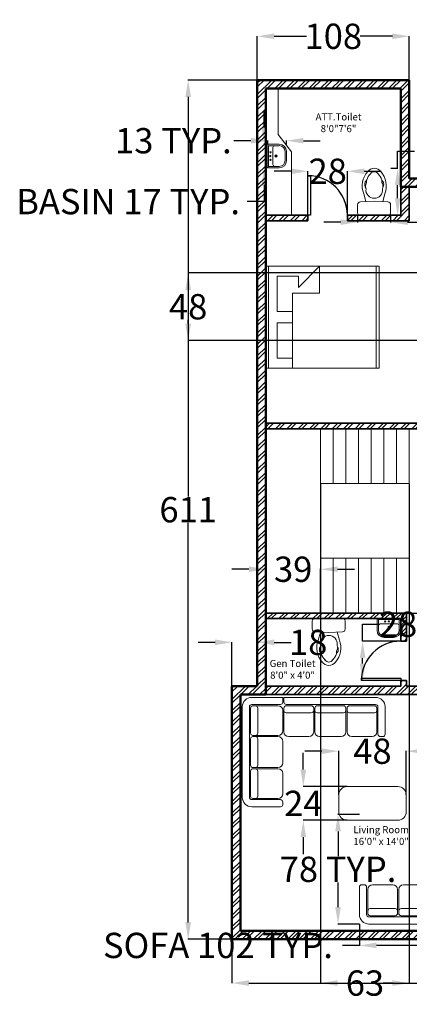
# Model space of a CAD drawing. Units: inches. Extents: x 7 to 752, y -275 to 426.
# Tile 1 of 5: x 7 to 284, y -275 to 426. Entities that reach past the tile are written whole.
import ezdxf

# ---------------------------------------------------------------- set-up
doc = ezdxf.new("R2010")
doc.units = ezdxf.units.IN
for name, color, linetype, lineweight in [('A-ANNO-DIMS', 2, 'Continuous', 18), ('A-AREA-IDEN', 7, 'Continuous', 18), ('A-DOOR', 6, 'Continuous', 25), ('A-FLOR-CASE', 2, 'Continuous', 18), ('A-FLOR-FIXT', 8, 'Continuous', 18), ('A-FLOR-STRS', 7, 'Continuous', 18), ('A-WALL-PATT', 252, 'Continuous', 13), ('Furniture', 2, 'Continuous', 18), ('Inner Wall', 5, 'Continuous', 35), ('Outer Wall', 1, 'Continuous', 50)]:
    doc.layers.add(name, color=color, linetype=linetype, lineweight=lineweight)
doc.styles.get("Standard").update_dxf_attribs({"font": 'arial.ttf'})
doc.dimstyles.get("Standard").update_dxf_attribs({"dimtxt": 18, "dimasz": 12, "dimexe": 0.18, "dimexo": 0.0625, "dimgap": 0.09, "dimtad": 0, "dimtih": 1, "dimtoh": 1, "dimdec": 0, "dimzin": 0, "dimdsep": 46, "dimlunit": 3, "dimtxsty": 'Standard', "dimcen": 0.09, "dimadec": 0, "dimazin": 0, "dimtfac": 1, "dimtdec": 0, "dimtofl": 0, "dimtmove": 0, "dimatfit": 3, "dimfxl": 1, "dimtolj": 1, "dimtzin": 0, "dimarcsym": 0})
pattern_1 = [(45, (-434.707, -1257.0093), (-4.041115, 4.041115), []), (45, (-432.013, -1257.0093), (-4.041115, 4.041115), [])]

# ---------------------------------------------------------------- blocks, each defined once
blk = doc.blocks.new('*U2')
for p, q in [((0, 0), (0, -4)), ((28, 0), (28, -4))]:
    blk.add_line(p, q)
blk.add_lwpolyline([(0, 0), (0, 28), (1.75, 28), (1.75, 0)], close=True)
blk.add_arc((0, 0), 28, 0, 90)
blk = doc.blocks.new('A$C2AFA021D')
for p, q in [((0.8, 2.3), (0.2, 2.3)), ((0, 2.1), (0, 0.2)), ((0.15, 0.2), (0.15, 2.1)), ((0.175, 1.55), (0.175, 2.075)), ((0.2, 2.15), (0.8, 2.15)), ((0.225, 2.125), (0.275, 2.125)), ((0.75, 2.125), (0.275, 2.125)), ((0.325, 2.075), (0.325, 1.55)), ((0.85, 2.2), (0.85, 2.25)), ((0.85, 1.6), (0.85, 2.025)), ((0.275, 1.5), (0.225, 1.5)), ((0.225, 1.475), (0.275, 1.475)), ((0.275, 1.5), (0.75, 1.5)), ((0.75, 1.475), (0.275, 1.475)), ((0.175, 0.875), (0.175, 1.425)), ((0.325, 1.425), (0.325, 0.875)), ((0.85, 0.925), (0.85, 1.375)), ((0.175, 0.225), (0.175, 0.75)), ((0.275, 0.825), (0.225, 0.825)), ((0.225, 0.8), (0.275, 0.8)), ((0.275, 0.825), (0.75, 0.825)), ((0.75, 0.8), (0.275, 0.8)), ((0.325, 0.75), (0.325, 0.225)), ((0.85, 0.275), (0.85, 0.7)), ((0.875, 0.275), (0.875, 0.725)), ((0.975, 0.825), (1.4, 0.825)), ((1.5, 0.725), (1.5, 0.275)), ((1.525, 0.275), (1.525, 0.725)), ((1.625, 0.825), (2.075, 0.825)), ((2.175, 0.725), (2.175, 0.275)), ((2.2, 0.275), (2.2, 0.725)), ((2.3, 0.825), (2.725, 0.825)), ((2.825, 0.725), (2.825, 0.275)), ((2.85, 0.2), (2.85, 0.775)), ((2.9, 0.825), (2.95, 0.825)), ((3, 0.775), (3, 0.2)), ((0.875, 0.275), (0.875, 0.225)), ((1.45, 0.325), (0.925, 0.325)), ((1.5, 0.225), (1.5, 0.275)), ((1.525, 0.275), (1.525, 0.225)), ((2.125, 0.325), (1.575, 0.325)), ((2.175, 0.225), (2.175, 0.275)), ((2.2, 0.275), (2.2, 0.225)), ((2.775, 0.325), (2.25, 0.325)), ((2.825, 0.225), (2.825, 0.275)), ((0.8, 0.15), (0.2, 0.15)), ((0.275, 0.175), (0.225, 0.175)), ((0.275, 0.175), (0.75, 0.175)), ((0.85, 0), (0.85, 0.1)), ((0.875, 0.1), (0.875, 0)), ((0.925, 0.175), (1.45, 0.175)), ((0.925, 0.15), (2.8, 0.15)), ((1.575, 0.175), (2.125, 0.175)), ((2.25, 0.175), (2.775, 0.175)), ((0.2, 0), (0.85, 0)), ((2.8, 0), (0.875, 0))]:
    blk.add_line(p, q)
for centre, radius, start, end in [((0.2, 2.1), 0.2, 90, 180), ((0.8, 2.25), 0.05, 0, 90), ((0.2, 2.1), 0.05, 90, 180), ((0.225, 2.075), 0.05, 90, 180), ((0.275, 2.075), 0.05, 0, 90), ((0.75, 2.025), 0.1, 0, 90), ((0.8, 2.2), 0.05, 270, 0), ((0.225, 1.55), 0.05, 180, 270), ((0.225, 1.425), 0.05, 90, 180), ((0.275, 1.55), 0.05, 270, 0), ((0.275, 1.425), 0.05, 0, 90), ((0.75, 1.6), 0.1, 270, 0), ((0.75, 1.375), 0.1, 360, 90), ((0.225, 0.875), 0.05, 180, 270), ((0.275, 0.875), 0.05, 270, 0), ((0.75, 0.925), 0.1, 270, 0), ((0.225, 0.75), 0.05, 90, 180), ((0.275, 0.75), 0.05, 0, 90), ((0.75, 0.7), 0.1, 0, 90), ((0.975, 0.725), 0.1, 90, 180), ((1.4, 0.725), 0.1, 0, 90), ((1.625, 0.725), 0.1, 90, 180), ((2.075, 0.725), 0.1, 0, 90), ((2.3, 0.725), 0.1, 90, 180), ((2.725, 0.725), 0.1, 0, 90), ((2.9, 0.775), 0.05, 90, 180), ((2.95, 0.775), 0.05, 0, 90), ((0.225, 0.225), 0.05, 180, 270), ((0.275, 0.225), 0.05, 270, 0), ((0.75, 0.275), 0.1, 270, 0), ((0.925, 0.275), 0.05, 90, 180), ((0.925, 0.225), 0.05, 180, 270), ((1.45, 0.275), 0.05, 360, 90), ((1.45, 0.225), 0.05, 270, 0), ((1.575, 0.275), 0.05, 90, 180), ((1.575, 0.225), 0.05, 180, 270), ((2.125, 0.275), 0.05, 360, 90), ((2.125, 0.225), 0.05, 270, 0), ((2.25, 0.275), 0.05, 90, 180), ((2.25, 0.225), 0.05, 180, 270), ((2.775, 0.275), 0.05, 360, 90), ((2.775, 0.225), 0.05, 270, 0), ((0.2, 0.2), 0.2, 180, 270), ((0.2, 0.2), 0.05, 180, 270), ((0.8, 0.1), 0.05, 0, 90), ((0.925, 0.1), 0.05, 90, 180), ((2.8, 0.2), 0.2, 270, 0), ((2.8, 0.2), 0.05, 270, 0)]:
    blk.add_arc(centre, radius, start, end)
blk = doc.blocks.new('A$C1308471B')
at = {"ltscale": 20}
for p, q in [((0, 0.461), (0, 0.019)), ((0.035, 0.479), (0.15, 0.479)), ((0.201, 0.24), (0.192, 0.438)), ((0.196, 0.364), (0.311, 0.395)), ((0.502, 0.353), (0.472, 0.353)), ((0.498, 0.357), (0.482, 0.371)), ((0.201, 0.24), (0.192, 0.041)), ((0.035, 0), (0.15, 0)), ((0.196, 0.119), (0.311, 0.088)), ((0.502, 0.13), (0.472, 0.13)), ((0.498, 0.126), (0.482, 0.112))]:
    blk.add_line(p, q, dxfattribs=at)
for centre, radius, start, end in [((0.006, 0.461), 0.006, 136.5269, 180), ((0.035, 0.433), 0.0465, 90, 136.5269), ((0.15, 0.436), 0.0429, 2.5755, 90), ((0.365, 0.242), 0.121, 83.3523, 180), ((0.425, 0.11), 0.307, 47.4135, 111.7924), ((0.382, 0.387), 0.0255, 263.3523, 298.5742), ((0.449, 0.264), 0.115, 79.3968, 118.5742), ((0.405, 0.216), 0.153, 63.502, 90.4522), ((0.466, 0.351), 0.0255, 50, 79.3968), ((0.515, 0.377), 0.0255, 230, 251.3881), ((0.502, 0.327), 0.0255, 70.3751, 90), ((0.425, 0.11), 0.256, 46.612, 70.3751), ((0.565, 0.242), 0.065, 0, 57.2974), ((0.565, 0.242), 0.116, 0, 54.7115), ((0.365, 0.242), 0.121, 180, 276.6477), ((0.425, 0.373), 0.307, 248.2076, 312.5865), ((0.425, 0.373), 0.256, 289.6249, 313.388), ((0.565, 0.242), 0.065, 302.7026, 0), ((0.565, 0.242), 0.116, 305.2885, 0), ((0.006, 0.019), 0.006, 180, 223.4731), ((0.035, 0.047), 0.0465, 223.4731, 270), ((0.15, 0.043), 0.0429, 270, 357.4245), ((0.382, 0.096), 0.0255, 61.4258, 96.6477), ((0.449, 0.22), 0.115, 241.4258, 280.6032), ((0.405, 0.267), 0.153, 269.5478, 296.498), ((0.466, 0.132), 0.0255, 280.6032, 310), ((0.515, 0.106), 0.0255, 108.6119, 130), ((0.502, 0.156), 0.0255, 270, 289.6249)]:
    blk.add_arc(centre, radius, start, end, dxfattribs=at)
blk = doc.blocks.new('A$C57EA129C')
for p, q in [((0, 0.443), (0, 0.178)), ((0.016, 0.459), (0.563, 0.459)), ((0.036, 0.432), (0.036, 0.29)), ((0.036, 0.29), (0.036, 0.178)), ((0.045, 0.441), (0.535, 0.441)), ((0.08, 0.334), (0.499, 0.334)), ((0.544, 0.432), (0.544, 0.29)), ((0.544, 0.29), (0.544, 0.178)), ((0.579, 0.443), (0.579, 0.178)), ((0.178, 0.036), (0.401, 0.036)), ((0.178, 0), (0.401, 0))]:
    blk.add_line(p, q)
for centre, radius in [((0.198, 0.392), 0.0143), ((0.29, 0.255), 0.0267), ((0.29, 0.255), 0.0178), ((0.29, 0.396), 0.0156), ((0.381, 0.392), 0.0143)]:
    blk.add_circle(centre, radius)
for centre, radius, start, end in [((0.016, 0.443), 0.016, 90, 180), ((0.045, 0.432), 0.00891, 90, 180), ((0.08, 0.29), 0.0445, 90, 180), ((0.499, 0.29), 0.0445, 0, 90), ((0.535, 0.432), 0.00891, 0, 90), ((0.563, 0.443), 0.016, 0, 90), ((0.178, 0.178), 0.178, 180, 270), ((0.178, 0.178), 0.143, 180, 270), ((0.401, 0.178), 0.178, 270, 0), ((0.401, 0.178), 0.143, 270, 0)]:
    blk.add_arc(centre, radius, start, end)
blk = doc.blocks.new('KING-00')
for p, q in [((-0.897, -0.947), (-0.897, 0.882)), ((0.602, 0.882), (0.602, -0.464)), ((1.034, -0.947), (1.034, 0.882)), ((0.602, 0.704), (0.881, 0.704)), ((0.881, 0.069), (0.881, 0.704)), ((0.602, 0.069), (0.881, 0.069)), ((0.881, -0.134), (0.602, -0.134)), ((0.881, -0.769), (0.881, -0.134)), ((0.119, -0.464), (0.119, -0.947)), ((0.602, -0.464), (0.119, -0.464)), ((0.119, -0.947), (0.5, -0.566)), ((0.5, -0.769), (0.5, -0.566)), ((0.5, -0.769), (0.881, -0.769))]:
    blk.add_line(p, q)
blk.add_lwpolyline([(-0.948, -0.947), (-0.948, 0.882), (1.084, 0.882), (1.084, -0.947)], close=True)
blk = doc.blocks.new('*D14')
at = {"layer": 'A-ANNO-DIMS', "color": 0, "lineweight": -2, "transparency": 16777216}
for p, q in [((181.23, 349.07), (181.23, 361.07)), ((183.68, 337.07), (181.05, 337.07)), ((183.68, 320.28), (181.05, 320.28)), ((181.23, 308.28), (181.23, 296.28)), ((181.23, 296.28), (169.23, 296.28))]:
    blk.add_line(p, q, dxfattribs=at)
at = {"layer": 'A-ANNO-DIMS', "color": 0, "transparency": 16777216}
for points in [[(179.23, 349.07), (183.23, 349.07), (181.23, 337.07)], [(179.23, 308.28), (183.23, 308.28), (181.23, 320.28)]]:
    blk.add_solid(points, dxfattribs=at)
at = {"layer": 'Defpoints', "color": 0, "transparency": 16777216}
for p in [(183.75, 337.07), (181.23, 320.28), (183.75, 320.28)]:
    blk.add_point(p, dxfattribs=at)
at = {"layer": 'A-ANNO-DIMS', "color": 0, "transparency": 16777216, "insert": (84.5, 296.28), "char_height": 18, "attachment_point": 5}
blk.add_mtext('\\A1;BASIN 17 TYP.', dxfattribs=at)
blk = doc.blocks.new('*D15')
at = {"layer": 'A-ANNO-DIMS', "color": 0, "lineweight": -2, "transparency": 16777216}
for p, q in [((171.75, 339.58), (159.75, 339.58)), ((183.75, 337.13), (183.75, 339.76)), ((197.05, 337.13), (197.05, 339.76)), ((209.05, 339.58), (221.05, 339.58))]:
    blk.add_line(p, q, dxfattribs=at)
at = {"layer": 'A-ANNO-DIMS', "color": 0, "transparency": 16777216}
for points in [[(171.75, 341.58), (171.75, 337.58), (183.75, 339.58)], [(209.05, 341.58), (209.05, 337.58), (197.05, 339.58)]]:
    blk.add_solid(points, dxfattribs=at)
at = {"layer": 'Defpoints', "color": 0, "transparency": 16777216}
for p in [(183.75, 339.58), (183.75, 337.07), (197.05, 337.07)]:
    blk.add_point(p, dxfattribs=at)
at = {"layer": 'A-ANNO-DIMS', "color": 0, "transparency": 16777216, "insert": (116.69, 339.58), "char_height": 18, "attachment_point": 5}
blk.add_mtext('\\A1;13 TYP.', dxfattribs=at)
blk = doc.blocks.new('*D16')
at = {"layer": 'A-ANNO-DIMS', "color": 0, "lineweight": -2, "transparency": 16777216}
for p, q in [((276.06, 320.03), (276.06, 332.03)), ((276.06, 332.03), (288.06, 332.03)), ((271.12, 320.03), (276.24, 320.03)), ((276.06, 298.68), (276.06, 308.03)), ((271.12, 286.68), (276.24, 286.68))]:
    blk.add_line(p, q, dxfattribs=at)
at = {"layer": 'A-ANNO-DIMS', "color": 0, "transparency": 16777216}
for points in [[(274.06, 308.03), (278.06, 308.03), (276.06, 320.03)], [(274.06, 298.68), (278.06, 298.68), (276.06, 286.68)]]:
    blk.add_solid(points, dxfattribs=at)
at = {"layer": 'Defpoints', "color": 0, "transparency": 16777216}
for p in [(271.06, 320.03), (276.06, 320.03), (271.06, 286.68)]:
    blk.add_point(p, dxfattribs=at)
at = {"layer": 'A-ANNO-DIMS', "color": 0, "transparency": 16777216, "insert": (356.77, 332.03), "char_height": 18, "attachment_point": 5}
blk.add_mtext('\\A1;WC 33 TYP.', dxfattribs=at)
blk = doc.blocks.new('*D17')
at = {"layer": 'A-ANNO-DIMS', "color": 0, "lineweight": -2, "transparency": 16777216}
for p, q in [((235.6, 281.67), (223.6, 281.67)), ((247.6, 286.61), (247.6, 281.49)), ((271.06, 286.61), (271.06, 281.49)), ((283.06, 281.67), (295.06, 281.67))]:
    blk.add_line(p, q, dxfattribs=at)
at = {"layer": 'A-ANNO-DIMS', "color": 0, "transparency": 16777216}
for points in [[(235.6, 283.67), (235.6, 279.67), (247.6, 281.67)], [(283.06, 283.67), (283.06, 279.67), (271.06, 281.67)]]:
    blk.add_solid(points, dxfattribs=at)
at = {"layer": 'Defpoints', "color": 0, "transparency": 16777216}
for p in [(247.6, 286.68), (271.06, 286.68), (271.06, 281.67)]:
    blk.add_point(p, dxfattribs=at)
at = {"layer": 'A-ANNO-DIMS', "color": 0, "transparency": 16777216, "insert": (339.11, 281.67), "char_height": 18, "attachment_point": 5}
blk.add_mtext('\\A1;23 TYP.', dxfattribs=at)
blk = doc.blocks.new('*D18')
at = {"layer": 'A-ANNO-DIMS', "color": 0, "lineweight": -2, "transparency": 16777216}
for p, q in [((248.92, -217.54), (248.92, -232.89)), ((350.44, -217.54), (350.44, -232.89)), ((248.92, -232.71), (236.92, -232.71)), ((338.44, -232.71), (260.92, -232.71))]:
    blk.add_line(p, q, dxfattribs=at)
at = {"layer": 'A-ANNO-DIMS', "color": 0, "transparency": 16777216}
for points in [[(260.92, -230.71), (260.92, -234.71), (248.92, -232.71)], [(338.44, -230.71), (338.44, -234.71), (350.44, -232.71)]]:
    blk.add_solid(points, dxfattribs=at)
at = {"layer": 'Defpoints', "color": 0, "transparency": 16777216}
for p in [(248.92, -217.48), (350.44, -217.48), (248.92, -232.71)]:
    blk.add_point(p, dxfattribs=at)
at = {"layer": 'A-ANNO-DIMS', "color": 0, "transparency": 16777216, "insert": (148.35, -232.71), "char_height": 18, "attachment_point": 5}
blk.add_mtext('\\A1;SOFA 102 TYP.', dxfattribs=at)
blk = doc.blocks.new('*D19')
at = {"layer": 'A-ANNO-DIMS', "color": 0, "lineweight": -2, "transparency": 16777216}
for p, q in [((248.86, -139.65), (233.51, -139.65)), ((233.69, -151.65), (233.69, -169.29)), ((233.69, -205.48), (233.69, -187.85)), ((248.86, -217.48), (233.51, -217.48))]:
    blk.add_line(p, q, dxfattribs=at)
at = {"layer": 'A-ANNO-DIMS', "color": 0, "transparency": 16777216}
for points in [[(231.69, -151.65), (235.69, -151.65), (233.69, -139.65)], [(231.69, -205.48), (235.69, -205.48), (233.69, -217.48)]]:
    blk.add_solid(points, dxfattribs=at)
at = {"layer": 'Defpoints', "color": 0, "transparency": 16777216}
for p in [(233.69, -139.65), (248.92, -139.65), (248.92, -217.48)]:
    blk.add_point(p, dxfattribs=at)
at = {"layer": 'A-ANNO-DIMS', "color": 0, "transparency": 16777216, "insert": (233.69, -178.57), "char_height": 18, "attachment_point": 5}
blk.add_mtext('\\A1;78 TYP.', dxfattribs=at)
blk = doc.blocks.new('*D30')
at = {"layer": 'A-ANNO-DIMS', "color": 0, "lineweight": -2, "transparency": 16777216}
for p, q in [((626.33, -52.39), (626.33, -259.65)), ((158.33, -228.39), (158.33, -259.65)), ((170.33, -259.47), (371.97, -259.47)), ((614.33, -259.47), (412.68, -259.47))]:
    blk.add_line(p, q, dxfattribs=at)
at = {"layer": 'A-ANNO-DIMS', "color": 0, "transparency": 16777216}
for points in [[(170.33, -257.47), (170.33, -261.47), (158.33, -259.47)], [(614.33, -257.47), (614.33, -261.47), (626.33, -259.47)]]:
    blk.add_solid(points, dxfattribs=at)
at = {"layer": 'Defpoints', "color": 0, "transparency": 16777216}
for p in [(626.33, -52.32), (158.33, -228.32), (626.33, -259.47)]:
    blk.add_point(p, dxfattribs=at)
at = {"layer": 'A-ANNO-DIMS', "color": 0, "transparency": 16777216, "insert": (392.33, -259.47), "char_height": 18, "attachment_point": 5}
blk.add_mtext('\\A1;468', dxfattribs=at)
blk = doc.blocks.new('*D31')
at = {"layer": 'A-ANNO-DIMS', "color": 0, "lineweight": -2, "transparency": 16777216}
for p, q in [((176.27, 382.68), (127, 382.68)), ((127.18, 370.68), (127.18, 86.46)), ((127.18, -216.32), (127.18, 67.9)), ((158.27, -228.32), (127, -228.32))]:
    blk.add_line(p, q, dxfattribs=at)
at = {"layer": 'A-ANNO-DIMS', "color": 0, "transparency": 16777216}
for points in [[(125.18, 370.68), (129.18, 370.68), (127.18, 382.68)], [(125.18, -216.32), (129.18, -216.32), (127.18, -228.32)]]:
    blk.add_solid(points, dxfattribs=at)
at = {"layer": 'Defpoints', "color": 0, "transparency": 16777216}
for p in [(127.18, 382.68), (176.33, 382.68), (158.33, -228.32)]:
    blk.add_point(p, dxfattribs=at)
at = {"layer": 'A-ANNO-DIMS', "color": 0, "transparency": 16777216, "insert": (127.18, 77.18), "char_height": 18, "attachment_point": 5}
blk.add_mtext('\\A1;611', dxfattribs=at)
blk = doc.blocks.new('*D32')
at = {"layer": 'A-ANNO-DIMS', "color": 0, "lineweight": -2, "transparency": 16777216}
for p, q in [((146.33, -17.17), (134.33, -17.17)), ((158.33, -48.26), (158.33, -16.99)), ((176.33, -48.26), (176.33, -16.99)), ((188.33, -17.17), (200.33, -17.17))]:
    blk.add_line(p, q, dxfattribs=at)
at = {"layer": 'A-ANNO-DIMS', "color": 0, "transparency": 16777216}
for points in [[(146.33, -15.17), (146.33, -19.17), (158.33, -17.17)], [(188.33, -15.17), (188.33, -19.17), (176.33, -17.17)]]:
    blk.add_solid(points, dxfattribs=at)
at = {"layer": 'Defpoints', "color": 0, "transparency": 16777216}
for p in [(176.33, -17.17), (158.33, -48.32), (176.33, -48.32)]:
    blk.add_point(p, dxfattribs=at)
at = {"layer": 'A-ANNO-DIMS', "color": 0, "transparency": 16777216, "insert": (212.48, -17.17), "char_height": 18, "attachment_point": 5}
blk.add_mtext('\\A1;18', dxfattribs=at)
blk = doc.blocks.new('*D33')
at = {"layer": 'A-ANNO-DIMS', "color": 0, "lineweight": -2, "transparency": 16777216}
for p, q in [((176.33, 382.74), (176.33, 414.01)), ((188.33, 413.83), (211.18, 413.83)), ((272.33, 413.83), (249.47, 413.83)), ((284.33, 382.74), (284.33, 414.01))]:
    blk.add_line(p, q, dxfattribs=at)
at = {"layer": 'A-ANNO-DIMS', "color": 0, "transparency": 16777216}
for points in [[(188.33, 415.83), (188.33, 411.83), (176.33, 413.83)], [(272.33, 415.83), (272.33, 411.83), (284.33, 413.83)]]:
    blk.add_solid(points, dxfattribs=at)
at = {"layer": 'Defpoints', "color": 0, "transparency": 16777216}
for p in [(284.33, 413.83), (176.33, 382.68), (284.33, 382.68)]:
    blk.add_point(p, dxfattribs=at)
at = {"layer": 'A-ANNO-DIMS', "color": 0, "transparency": 16777216, "insert": (230.33, 413.83), "char_height": 18, "attachment_point": 5}
blk.add_mtext('\\A1;108', dxfattribs=at)
blk = doc.blocks.new('*D41')
at = {"layer": 'A-ANNO-DIMS', "color": 0, "lineweight": -2, "transparency": 16777216}
for p, q in [((170.328243, 34.826615), (158.328243, 34.826615)), ((182.328243, 3.739115), (182.328243, 35.006615)), ((221.328243, 3.739115), (221.328243, 35.006615)), ((233.328243, 34.826615), (245.328243, 34.826615))]:
    blk.add_line(p, q, dxfattribs=at)
at = {"layer": 'A-ANNO-DIMS', "color": 0, "transparency": 16777216}
for points in [[(170.328243, 36.826615), (170.328243, 32.826615), (182.328243, 34.826615)], [(233.328243, 36.826615), (233.328243, 32.826615), (221.328243, 34.826615)]]:
    blk.add_solid(points, dxfattribs=at)
at = {"layer": 'Defpoints', "color": 0, "transparency": 16777216}
for p in [(221.328243, 34.826615), (182.328243, 3.676615), (221.328243, 3.676615)]:
    blk.add_point(p, dxfattribs=at)
at = {"layer": 'A-ANNO-DIMS', "color": 0, "transparency": 16777216, "insert": (201.828243, 34.826615), "char_height": 18, "attachment_point": 5}
blk.add_mtext('\\A1;39', dxfattribs=at)
blk = doc.blocks.new('*D42')
at = {"layer": 'A-ANNO-DIMS', "color": 0, "lineweight": -2, "transparency": 16777216}
for p, q in [((221.33, 95.61), (221.33, -259.65)), ((284.33, 95.61), (284.33, -259.65)), ((233.33, -259.47), (239.8, -259.47)), ((272.33, -259.47), (265.86, -259.47))]:
    blk.add_line(p, q, dxfattribs=at)
at = {"layer": 'A-ANNO-DIMS', "color": 0, "transparency": 16777216}
for points in [[(233.33, -257.47), (233.33, -261.47), (221.33, -259.47)], [(272.33, -257.47), (272.33, -261.47), (284.33, -259.47)]]:
    blk.add_solid(points, dxfattribs=at)
at = {"layer": 'Defpoints', "color": 0, "transparency": 16777216}
for p in [(221.33, 95.68), (284.33, 95.68), (284.33, -259.47)]:
    blk.add_point(p, dxfattribs=at)
at = {"layer": 'A-ANNO-DIMS', "color": 0, "transparency": 16777216, "insert": (252.83, -259.47), "char_height": 18, "attachment_point": 5}
blk.add_mtext('\\A1;63', dxfattribs=at)
blk = doc.blocks.new('*D43')
at = {"layer": 'A-ANNO-DIMS', "color": 0, "lineweight": -2, "transparency": 16777216}
for p, q in [((221.39, 134.68), (657.66, 134.68)), ((657.48, 122.68), (657.48, 78.46)), ((657.48, 15.68), (657.48, 59.89)), ((221.39, 3.68), (657.66, 3.68))]:
    blk.add_line(p, q, dxfattribs=at)
at = {"layer": 'A-ANNO-DIMS', "color": 0, "transparency": 16777216}
for points in [[(655.48, 122.68), (659.48, 122.68), (657.48, 134.68)], [(655.48, 15.68), (659.48, 15.68), (657.48, 3.68)]]:
    blk.add_solid(points, dxfattribs=at)
at = {"layer": 'Defpoints', "color": 0, "transparency": 16777216}
for p in [(221.33, 134.68), (657.48, 134.68), (221.33, 3.68)]:
    blk.add_point(p, dxfattribs=at)
at = {"layer": 'A-ANNO-DIMS', "color": 0, "transparency": 16777216, "insert": (657.48, 69.18), "char_height": 18, "attachment_point": 5}
blk.add_mtext('\\A1;131', dxfattribs=at)
blk = doc.blocks.new('*D47')
at = {"layer": 'A-ANNO-DIMS', "color": 0, "lineweight": -2, "transparency": 16777216}
for p, q in [((520.1, 245.5), (127, 245.5)), ((127.18, 233.5), (127.18, 230.78)), ((127.18, 209.5), (127.18, 212.22)), ((520.1, 197.5), (127, 197.5))]:
    blk.add_line(p, q, dxfattribs=at)
at = {"layer": 'A-ANNO-DIMS', "color": 0, "transparency": 16777216}
for points in [[(125.18, 233.5), (129.18, 233.5), (127.18, 245.5)], [(125.18, 209.5), (129.18, 209.5), (127.18, 197.5)]]:
    blk.add_solid(points, dxfattribs=at)
at = {"layer": 'Defpoints', "color": 0, "transparency": 16777216}
for p in [(127.18, 245.5), (520.16, 245.5), (520.16, 197.5)]:
    blk.add_point(p, dxfattribs=at)
at = {"layer": 'A-ANNO-DIMS', "color": 0, "transparency": 16777216, "insert": (127.18, 221.5), "char_height": 18, "attachment_point": 5}
blk.add_mtext('\\A1;48', dxfattribs=at)
blk = doc.blocks.new('*D51')
at = {"layer": 'A-ANNO-DIMS', "color": 0, "lineweight": -2, "transparency": 16777216}
for p, q in [((200.328243, 317.826615), (188.328243, 317.826615)), ((212.328243, 286.739115), (212.328243, 318.006615)), ((240.328243, 286.739115), (240.328243, 318.006615)), ((252.328243, 317.826615), (264.328243, 317.826615))]:
    blk.add_line(p, q, dxfattribs=at)
at = {"layer": 'A-ANNO-DIMS', "color": 0, "transparency": 16777216}
for points in [[(200.328243, 319.826615), (200.328243, 315.826615), (212.328243, 317.826615)], [(252.328243, 319.826615), (252.328243, 315.826615), (240.328243, 317.826615)]]:
    blk.add_solid(points, dxfattribs=at)
at = {"layer": 'Defpoints', "color": 0, "transparency": 16777216}
for p in [(240.328243, 317.826615), (212.328243, 286.676615), (240.328243, 286.676615)]:
    blk.add_point(p, dxfattribs=at)
at = {"layer": 'A-ANNO-DIMS', "color": 0, "transparency": 16777216, "insert": (226.328243, 317.826615), "char_height": 18, "attachment_point": 5}
blk.add_mtext('\\A1;28', dxfattribs=at)
blk = doc.blocks.new('*D60')
at = {"layer": 'A-ANNO-DIMS', "color": 0, "lineweight": -2, "transparency": 16777216}
for p, q in [((222.170767, -94.562838), (210.170767, -94.562838)), ((234.170767, -125.650338), (234.170767, -94.382838)), ((282.170767, -125.650338), (282.170767, -94.382838)), ((294.170767, -94.562838), (306.170767, -94.562838))]:
    blk.add_line(p, q, dxfattribs=at)
at = {"layer": 'A-ANNO-DIMS', "color": 0, "transparency": 16777216}
for points in [[(222.170767, -92.562838), (222.170767, -96.562838), (234.170767, -94.562838)], [(294.170767, -92.562838), (294.170767, -96.562838), (282.170767, -94.562838)]]:
    blk.add_solid(points, dxfattribs=at)
at = {"layer": 'Defpoints', "color": 0, "transparency": 16777216}
for p in [(282.170767, -94.562838), (234.170767, -125.712838), (282.170767, -125.712838)]:
    blk.add_point(p, dxfattribs=at)
at = {"layer": 'A-ANNO-DIMS', "color": 0, "transparency": 16777216, "insert": (258.170767, -94.562838), "char_height": 18, "attachment_point": 5}
blk.add_mtext('\\A1;48', dxfattribs=at)
blk = doc.blocks.new('*D61')
at = {"layer": 'A-ANNO-DIMS', "color": 0, "lineweight": -2, "transparency": 16777216}
for p, q in [((209.020767, -107.712838), (209.020767, -95.712838)), ((240.108267, -119.712838), (208.840767, -119.712838)), ((240.108267, -143.712838), (208.840767, -143.712838)), ((209.020767, -155.712838), (209.020767, -167.712838))]:
    blk.add_line(p, q, dxfattribs=at)
at = {"layer": 'A-ANNO-DIMS', "color": 0, "transparency": 16777216}
for points in [[(207.020767, -107.712838), (211.020767, -107.712838), (209.020767, -119.712838)], [(207.020767, -155.712838), (211.020767, -155.712838), (209.020767, -143.712838)]]:
    blk.add_solid(points, dxfattribs=at)
at = {"layer": 'Defpoints', "color": 0, "transparency": 16777216}
for p in [(209.020767, -119.712838), (240.170767, -119.712838), (240.170767, -143.712838)]:
    blk.add_point(p, dxfattribs=at)
at = {"layer": 'A-ANNO-DIMS', "color": 0, "transparency": 16777216, "insert": (209.020767, -131.712838), "char_height": 18, "attachment_point": 5}
blk.add_mtext('\\A1;24', dxfattribs=at)
blk = doc.blocks.new('*D63')
at = {"layer": 'A-ANNO-DIMS', "color": 0, "lineweight": -2, "transparency": 16777216}
for p, q in [((251.18, -16.32), (251.18, -4.32)), ((251.18, -4.32), (263.18, -4.32)), ((282.27, -16.32), (251, -16.32)), ((251.18, -32.32), (251.18, -28.32)), ((282.27, -44.32), (251, -44.32))]:
    blk.add_line(p, q, dxfattribs=at)
at = {"layer": 'A-ANNO-DIMS', "color": 0, "transparency": 16777216}
for points in [[(249.18, -28.32), (253.18, -28.32), (251.18, -16.32)], [(249.18, -32.32), (253.18, -32.32), (251.18, -44.32)]]:
    blk.add_solid(points, dxfattribs=at)
at = {"layer": 'Defpoints', "color": 0, "transparency": 16777216}
for p in [(251.18, -16.32), (282.33, -16.32), (282.33, -44.32)]:
    blk.add_point(p, dxfattribs=at)
at = {"layer": 'A-ANNO-DIMS', "color": 0, "transparency": 16777216, "insert": (276.33, -4.32), "char_height": 18, "attachment_point": 5}
blk.add_mtext('\\A1;28', dxfattribs=at)

msp = doc.modelspace()

# ---------------------------------------------------------------- hatches: boundary and pattern name
at = {"layer": 'A-WALL-PATT'}
h = msp.add_hatch(dxfattribs=at)
h.set_pattern_fill('ANSI32', color=256, scale=0.6)
h.set_pattern_definition(pattern_1)
h.paths.add_polyline_path([(182.33, 376.68), (278.33, 376.68), (278.33, 306.68), (466.33, 306.68), (466.33, 312.68), (284.33, 312.68), (284.33, 382.68), (176.33, 382.68), (176.33, -48.32), (158.33, -48.32), (158.33, -228.32), (360.33, -228.32), (360.33, -137.32), (384.33, -137.32), (384.33, -131.32), (356.33, -131.32), (356.33, -222.32), (164.33, -222.32), (164.33, -54.32), (182.33, -54.32)])
h.paths.add_polyline_path([(626.33, 312.68), (502.33, 312.68), (502.33, 306.68), (620.33, 306.68), (620.33, 171.68), (620.33, -48.32), (544.33, -48.32), (544.33, -131.32), (432.33, -131.32), (432.33, -137.32), (550.33, -137.32), (550.33, -52.32), (626.33, -52.32)])
h = msp.add_hatch(dxfattribs=at)
h.set_pattern_fill('ANSI32', color=256, scale=0.6)
h.set_pattern_definition(pattern_1)
h.paths.add_polyline_path([(360.33, -48.32), (282.33, -48.32), (282.33, -44.32), (278.33, -44.32), (278.33, -48.32), (182.33, -48.32), (182.33, -54.32), (356.33, -54.32), (356.33, -89.32), (360.33, -89.32)])
h.paths.add_polyline_path([(484.33, -48.32), (460.33, -48.32), (460.33, -42.32), (456.33, -42.32), (456.33, -48.32), (432.33, -48.32), (432.33, -52.32), (456.33, -52.32), (456.33, -131.32), (460.33, -131.32), (460.33, -52.32), (484.33, -52.32)])
h.paths.add_polyline_path([(544.33, -48.32), (512.33, -48.32), (512.33, -52.32), (544.33, -52.32)])
h.paths.add_polyline_path([(460.33, 134.68), (484.33, 134.68), (620.33, 134.68), (620.33, 138.68), (460.33, 138.68), (460.33, 144.68), (456.33, 144.68), (456.33, -6.32), (460.33, -6.32)])
h.paths.add_polyline_path([(282.33, 3.68), (182.33, 3.68), (182.33, -0.32), (278.33, -0.32), (278.33, -16.32), (282.33, -16.32)])
h.paths.add_polyline_path([(378.33, 144.68), (374.33, 144.68), (374.33, 138.68), (182.33, 138.68), (182.33, 134.68), (378.33, 134.68)])
h.paths.add_polyline_path([(284.33, 306.68), (278.33, 306.68), (278.33, 286.68), (240.33, 286.68), (240.33, 282.68), (284.33, 282.68)])
h.paths.add_polyline_path([(212.33, 286.68), (182.33, 286.68), (182.33, 282.68), (212.33, 282.68)])
h.paths.add_polyline_path([(436.33, 225.08), (460.33, 225.08), (460.33, 229.08), (432.33, 229.08), (432.33, 184.68), (456.33, 184.68), (456.33, 180.68), (460.33, 180.68), (460.33, 188.68), (436.33, 188.68)])
h.paths.add_polyline_path([(432.33, 204.68), (378.33, 204.68), (378.33, 306.68), (374.33, 306.68), (374.33, 282.68), (374.33, 198.85), (374.33, 180.68), (378.33, 180.68), (378.33, 200.68), (432.33, 200.68)])
h.paths.add_polyline_path([(460.33, 270.68), (436.33, 270.68), (436.33, 306.68), (432.33, 306.68), (432.33, 282.68), (432.33, 266.68), (460.33, 266.68)])

# ---------------------------------------------------------------- linework, layer by layer
at = {"layer": 'A-FLOR-CASE'}
for p, q in [((191.25, 343.9), (191.25, 376.68)), ((200.56, 331.68), (191.25, 343.9)), ((200.56, 331.68), (200.56, 286.68))]:
    msp.add_line(p, q, dxfattribs=at)
at = {"layer": 'A-FLOR-STRS'}
for p, q in [((221.33, 134.68), (221.33, 3.68)), ((230.33, 134.68), (230.33, 95.68)), ((239.33, 134.68), (239.33, 95.68)), ((248.33, 134.68), (248.33, 95.68)), ((257.33, 134.68), (257.33, 95.68)), ((266.33, 134.68), (266.33, 95.68)), ((275.33, 134.68), (275.33, 95.68)), ((284.33, 134.68), (284.33, 95.68)), ((221.33, 95.68), (284.33, 95.68)), ((221.33, 42.68), (284.33, 42.68)), ((230.33, 42.68), (230.33, 3.68)), ((239.33, 42.68), (239.33, 3.68)), ((248.33, 42.68), (248.33, 3.68)), ((257.33, 42.68), (257.33, 3.68)), ((266.33, 42.68), (266.33, 3.68)), ((275.33, 42.68), (275.33, 3.68)), ((284.33, 42.68), (284.33, 3.68))]:
    msp.add_line(p, q, dxfattribs=at)
at = {"layer": 'Furniture'}
msp.add_lwpolyline([(234.17, -137.71), (234.17, -125.71, -0.414214), (240.17, -119.71), (276.17, -119.71, -0.414214), (282.17, -125.71), (282.17, -137.71, -0.414214), (276.17, -143.71), (240.17, -143.71, -0.414214)], format="xyb", close=True, dxfattribs=at)
at = {"layer": 'Inner Wall'}
for p, q in [((278.33, 286.68), (278.33, 306.68)), ((284.33, 306.68), (284.33, 282.68)), ((182.33, 286.68), (212.33, 286.68)), ((182.33, 282.68), (212.33, 282.68)), ((212.33, 286.68), (212.33, 282.68)), ((240.33, 286.68), (240.33, 282.68)), ((240.33, 286.68), (278.33, 286.68)), ((240.33, 282.68), (284.33, 282.68)), ((182.33, 138.68), (374.33, 138.68)), ((182.33, 134.68), (378.33, 134.68)), ((182.33, 3.68), (284.33, 3.68)), ((282.33, 3.68), (282.33, -16.32)), ((182.33, -0.32), (278.33, -0.32)), ((278.33, -0.32), (278.33, -16.32)), ((278.33, -16.32), (282.33, -16.32)), ((182.33, -48.32), (278.33, -48.32)), ((278.33, -44.32), (282.33, -44.32)), ((278.33, -44.32), (278.33, -48.32)), ((282.33, -44.32), (282.33, -48.32)), ((282.33, -48.32), (360.33, -48.32)), ((182.33, -54.32), (356.33, -54.32))]:
    msp.add_line(p, q, dxfattribs=at)
at = {"layer": 'Outer Wall'}
for p, q in [((176.33, 382.68), (176.33, -48.32)), ((176.33, 382.68), (284.33, 382.68)), ((284.33, 382.68), (284.33, 312.68)), ((182.33, 376.68), (182.33, -54.32)), ((182.33, 376.68), (278.33, 376.68)), ((278.33, 376.68), (278.33, 306.68)), ((466.33, 312.68), (284.33, 312.68)), ((278.33, 306.68), (466.33, 306.68)), ((158.33, -48.32), (176.33, -48.32)), ((158.33, -48.32), (158.33, -228.32)), ((164.33, -54.32), (164.33, -222.32)), ((164.33, -54.32), (182.33, -54.32)), ((164.33, -222.32), (356.33, -222.32)), ((158.33, -228.32), (360.33, -228.32))]:
    msp.add_line(p, q, dxfattribs=at)

# ---------------------------------------------------------------- block references
at = {"layer": 'A-DOOR'}
msp.add_blockref('*U2', (212.33, 286.68), dxfattribs=at)
at = {"layer": 'A-DOOR', "rotation": 89.99999999999999}
msp.add_blockref('*U2', (278.33, -44.32), dxfattribs=at)
at = {"layer": 'A-FLOR-FIXT'}
for name, p, xscale, yscale, zscale, rotation in [('A$C57EA129C', (197.05, 337.07), -28.98333223671166, 28.98333223671166, 28.98333223671166, 90), ('A$C1308471B', (247.6, 286.68), -48.95497407897215, 48.95497407897215, 48.95497407897215, 270.0000000000001), ('A$C1308471B', (215.32, -0.32), 48.95497407897215, 48.95497407897215, 48.95497407897215, 269.9999999999999)]:
    msp.add_blockref(name, p, dxfattribs=dict(at, xscale=xscale, yscale=yscale, zscale=zscale, rotation=rotation))
at = {"layer": 'A-FLOR-FIXT', "xscale": -28.98333223671166, "yscale": 28.98333223671166, "zscale": 28.98333223671166}
msp.add_blockref('A$C57EA129C', (278.2, -13.72), dxfattribs=at)
at = {"layer": 'Furniture', "rotation": 180}
for name, p, xscale, yscale, zscale in [('KING-00', (225.28, 212.83), 39.60249106241186, 39.60249106241186, 39.60249106241186), ('A$C2AFA021D', (165.63, -56.29), -33.84012530478223, 33.84012530478223, 33.84012530478223)]:
    msp.add_blockref(name, p, dxfattribs=dict(at, xscale=xscale, yscale=yscale, zscale=zscale))
at = {"layer": 'Furniture', "xscale": -33.84012530478223, "yscale": 33.84012530478223, "zscale": 33.84012530478223}
msp.add_blockref('A$C2AFA021D', (350.44, -217.48), dxfattribs=at)

# ---------------------------------------------------------------- texts
at = {"layer": 'A-AREA-IDEN', "char_height": 5, "attachment_point": 3}
for s, insert in [('\\pxqc;{\\fTimes New Roman|b0|i0|c0|p18;ATT.Toilet\\P8\'0"7\'6"}', (258.59, 359.01)), ('\\pxqc;{\\fTimes New Roman|b0|i0|c0|p18;Gen Toilet\\P8\'0" x 4\'0"}', (225.94, -29.69)), ('\\pxqc;{\\fTimes New Roman|b0|i0|c0|p18;Living Room\\P16\'0" x 14\'0"}', (288.88, -147.88))]:
    msp.add_mtext_dynamic_manual_height_columns(s, width=49.1019, gutter_width=12.5, heights=[0], dxfattribs=dict(at, insert=insert))

# ---------------------------------------------------------------- dimensions: what is measured, and where the dimension line sits
at = {"layer": 'A-ANNO-DIMS'}
for base, p1, p2, picture, middle in [((284.33, 413.83), (176.33, 382.68), (284.33, 382.68), '*D33', (230.33, 413.83)), ((240.33, 317.83), (212.33, 286.68), (240.33, 286.68), '*D51', (226.33, 317.83)), ((284.33, -259.47), (221.33, 95.68), (284.33, 95.68), '*D42', (252.83, -259.47)), ((176.33, -17.17), (158.33, -48.32), (176.33, -48.32), '*D32', (212.48, -17.17)), ((626.33, -259.47), (158.33, -228.32), (626.33, -52.32), '*D30', (392.33, -259.47)), ((282.17, -94.56), (234.17, -125.71), (282.17, -125.71), '*D60', (258.17, -94.56))]:
    dim = msp.add_linear_dim(base=base, p1=p1, p2=p2, dimstyle='Standard', override={"dimdec": 0, "dimlfac": 1, "dimrnd": 0, "dimzin": 0, "dimdsep": 46, "dimlunit": 2}, dxfattribs=at)
    dim.commit()
    dim.dimension.update_dxf_attribs({"geometry": picture, "text_midpoint": middle})
for base, p1, p2, angle, picture, middle in [((127.18, 382.68), (158.33, -228.32), (176.33, 382.68), 90, '*D31', (127.18, 77.18)), ((127.18, 245.5), (520.16, 197.5), (520.16, 245.5), 90, '*D47', (127.18, 221.5)), ((657.48, 134.68), (221.33, 3.68), (221.33, 134.68), 90, '*D43', (657.48, 69.18)), ((221.33, 34.83), (182.33, 3.68), (221.33, 3.68), 0, '*D41', (201.83, 34.83)), ((251.18, -16.32), (282.33, -44.32), (282.33, -16.32), 90, '*D63', (276.33, -4.32)), ((209.02, -119.71), (240.17, -143.71), (240.17, -119.71), 90, '*D61', (209.02, -131.71))]:
    dim = msp.add_linear_dim(base=base, p1=p1, p2=p2, angle=angle, dimstyle='Standard', override={"dimdec": 0, "dimlfac": 1, "dimrnd": 0, "dimzin": 0, "dimdsep": 46, "dimlunit": 2}, dxfattribs=at)
    dim.commit()
    dim.dimension.update_dxf_attribs({"geometry": picture, "text_midpoint": middle})
for base, p1, p2, angle, text, picture, middle in [((276.06, 320.03), (271.06, 286.68), (271.06, 320.03), 90, 'WC <> TYP.', '*D16', (356.77, 332.03)), ((183.75, 339.58), (197.05, 337.07), (183.75, 337.07), 180, '<> TYP.', '*D15', (116.69, 339.58)), ((181.23, 320.28), (183.75, 337.07), (183.75, 320.28), 270, 'BASIN <> TYP.', '*D14', (84.5, 296.28)), ((271.06, 281.67), (247.6, 286.68), (271.06, 286.68), 0, '<> TYP.', '*D17', (339.11, 281.67)), ((233.69, -139.65), (248.92, -217.48), (248.92, -139.65), 90, '<> TYP.', '*D19', (233.69, -178.57)), ((248.92, -232.71), (350.44, -217.48), (248.92, -217.48), 180, 'SOFA <> TYP.', '*D18', (148.35, -232.71))]:
    dim = msp.add_linear_dim(base=base, p1=p1, p2=p2, angle=angle, text=text, dimstyle='Standard', override={"dimdec": 0, "dimlfac": 1, "dimrnd": 0, "dimzin": 0, "dimdsep": 46, "dimlunit": 2}, dxfattribs=at)
    dim.commit()
    dim.dimension.update_dxf_attribs({"geometry": picture, "text_midpoint": middle})

doc.saveas('drawing.dxf')
